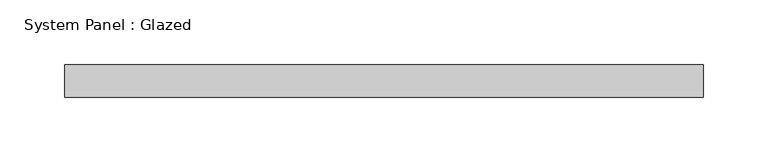
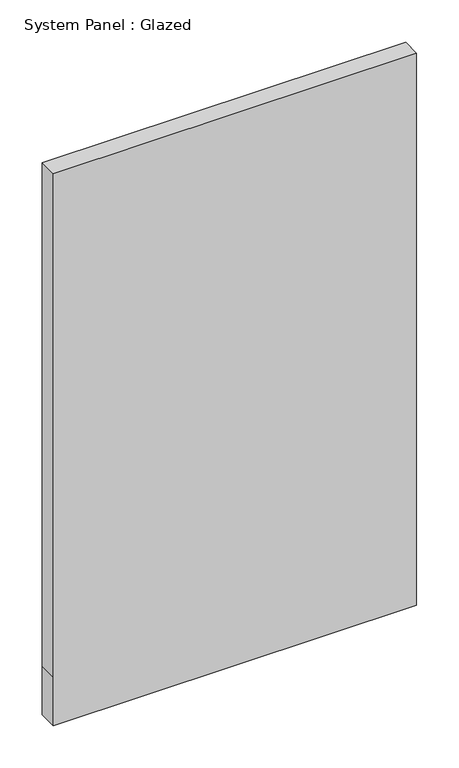
"""IFC4 building model written with IfcOpenShell, lengths in millimetres: plate geometry, System Panel : Glazed."""

from ifc_helpers import new_model, si_unit, frame, origin, place, context, project, spatial, polyline, outline, extrude, source, transform, mapped, element, save


def system_panel_glazed_713e3d92(model_context):
    return source(origin(), model_context, "Body", "SweptSolid", [
        extrude(outline(polyline([(0.0, -247.65), (0.0, 247.65), (69.85, 247.65), (794.5627727, 247.65), (794.5627727, -247.65), (69.85, -247.65), (0.0, -247.65)])), frame((0.0, 19.05, 0.0), z_axis=(0.0, 1.0, 0.0), x_axis=(0.0, 0.0, 1.0)), (0.0, 0.0, 1.0), 25.4),
    ])


if __name__ == "__main__":
    model = new_model("IFC4")
    model_context = context("Model", 3, world=origin())
    ifc_project = project(units=[si_unit("LENGTHUNIT", "METRE", prefix="MILLI")], contexts=[model_context])
    site = spatial("IfcSite", under=ifc_project)
    building = spatial("IfcBuilding", under=site)
    placement = place(None, origin())
    system_panel_glazed_shape = system_panel_glazed_713e3d92(model_context)
    element("IfcPlate", 1, ObjectType="System Panel : Glazed", at=placement, inside=building, context=model_context, shape_type="MappedRepresentation", body=[
        mapped(system_panel_glazed_shape, transform((0.0, 0.0, 0.0), x_axis=(1.0, 0.0, 0.0), y_axis=(0.0, 1.0, 0.0), z_axis=(0.0, 0.0, 1.0))),
    ])
    save(model, "model.ifc")

# Revit data of these elements
# Type "System Panel : Glazed"
#   Construction Type Id = "GSP4R"
#   Analytic Construction = "1/8 in Pilkington single glazing"
#   Visual Light Transmittance = 0.9
#   Solar Heat Gain Coefficient = 0.86
#   Heat Transfer Coefficient (U) = 1.18115 BTU/(h·ft²·°F)
#   Define Thermal Properties by = 1
# Element 1 (IfcPlate, "System Panel : Glazed")
#   Materials on its faces: "Glass"
# Materials
#   "Glass": class "Glass", colour RGB 0 128 192, transparency 0.75, Description = "Soda Lime Glass", Cost = 0
